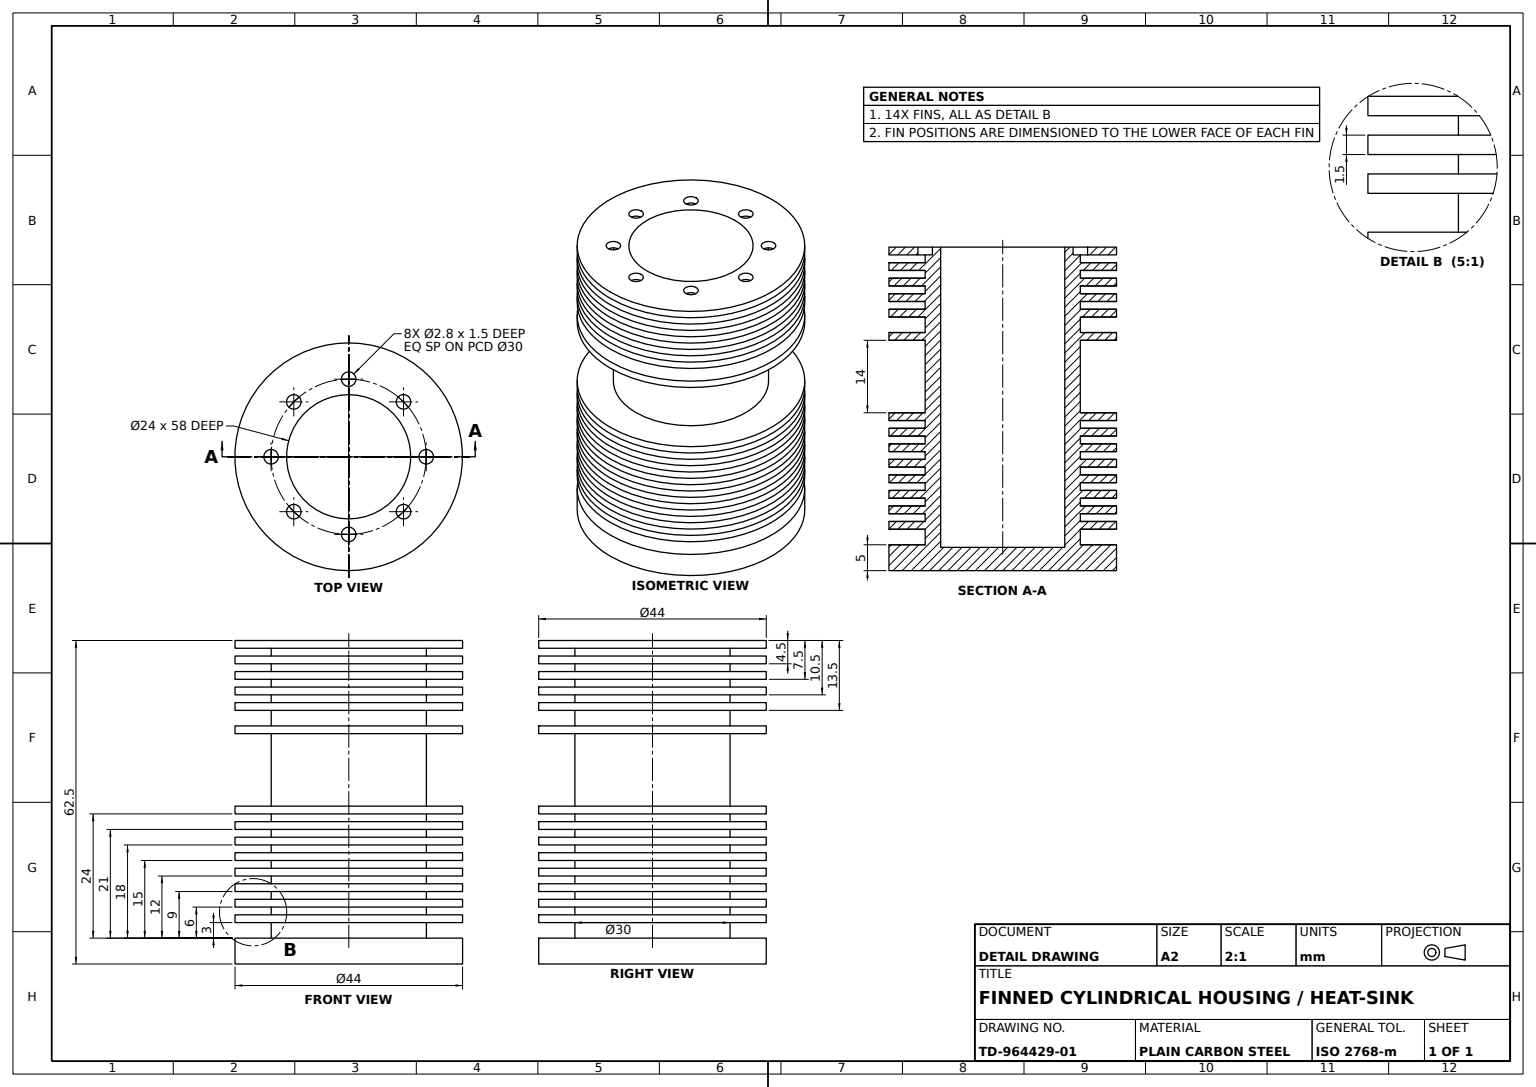
from build123d import *

# Parameters (mm, degrees)
BASE_DISC_SKETCH_R     = 22
BASE_DISC_DEPTH        = 5
LOWER_FIN_1_SKETCH_R   = 22
LOWER_FIN_1_DEPTH      = 1.5
LOWER_FIN_2_SKETCH_R   = 22
LOWER_FIN_2_DEPTH      = 1.5
LOWER_FIN_3_SKETCH_R   = 22
LOWER_FIN_3_DEPTH      = 1.5
LOWER_FIN_4_SKETCH_R   = 22
LOWER_FIN_4_DEPTH      = 1.5
LOWER_FIN_5_SKETCH_R   = 22
LOWER_FIN_5_DEPTH      = 1.5
LOWER_FIN_6_SKETCH_R   = 22
LOWER_FIN_6_DEPTH      = 1.5
LOWER_FIN_7_SKETCH_R   = 22
LOWER_FIN_7_DEPTH      = 1.5
LOWER_FIN_8_SKETCH_R   = 22
LOWER_FIN_8_DEPTH      = 1.5
UPPER_FIN_1_SKETCH_R   = 22
UPPER_FIN_1_DEPTH      = 1.5
UPPER_FIN_2_SKETCH_R   = 22
UPPER_FIN_2_DEPTH      = 1.5
UPPER_FIN_3_SKETCH_R   = 22
UPPER_FIN_3_DEPTH      = 1.5
UPPER_FIN_4_SKETCH_R   = 22
UPPER_FIN_4_DEPTH      = 1.5
UPPER_FIN_5_SKETCH_R   = 22
UPPER_FIN_5_DEPTH      = 1.5
UPPER_FIN_6_SKETCH_R   = 22
UPPER_FIN_6_DEPTH      = 1.5
CORE_BOSS_SKETCH_R     = 12
CORE_BOSS_58MM_DEPTH   = 58
HUB_BOSS_SKETCH_R      = 15
HUB_BOSS_58MM_DEPTH    = 58
CENTRAL_BORE_SKETCH_R  = 12
CENTRAL_BORE_DEPTH     = 58
BOLT_HOLES_8X_SKETCH_R = 1.4
BOLT_HOLES_8X_DEPTH    = 1.5


with BuildPart() as part:
    # Base Disc Sketch → Base Disc (new body)
    with BuildSketch(Plane(origin=(0, 0, 0), x_dir=(1, 0, 0), z_dir=(0, 1, 0))):
        with Locations(Location((0, 0, 0), (0, 0, 270))):
            Circle(BASE_DISC_SKETCH_R)
    extrude(amount=BASE_DISC_DEPTH)



with BuildPart() as body_2:
    # Lower Fin 1 Sketch → Lower Fin 1 (new body)
    with BuildSketch(Plane(origin=(0, 8, 0), x_dir=(1, 0, 0), z_dir=(0, 1, 0))):
        with Locations(Location((0, 0, 0), (0, 0, 270))):
            Circle(LOWER_FIN_1_SKETCH_R)
    extrude(amount=LOWER_FIN_1_DEPTH)


with BuildPart() as body_3:
    # Lower Fin 2 Sketch → Lower Fin 2 (new body)
    with BuildSketch(Plane(origin=(0, 11, 0), x_dir=(1, 0, 0), z_dir=(0, 1, 0))):
        with Locations(Location((0, 0, 0), (0, 0, 270))):
            Circle(LOWER_FIN_2_SKETCH_R)
    extrude(amount=LOWER_FIN_2_DEPTH)


with BuildPart() as body_4:
    # Lower Fin 3 Sketch → Lower Fin 3 (new body)
    with BuildSketch(Plane(origin=(0, 14, 0), x_dir=(1, 0, 0), z_dir=(0, 1, 0))):
        with Locations(Location((0, 0, 0), (0, 0, 270))):
            Circle(LOWER_FIN_3_SKETCH_R)
    extrude(amount=LOWER_FIN_3_DEPTH)


with BuildPart() as body_5:
    # Lower Fin 4 Sketch → Lower Fin 4 (new body)
    with BuildSketch(Plane(origin=(0, 17, 0), x_dir=(1, 0, 0), z_dir=(0, 1, 0))):
        with Locations(Location((0, 0, 0), (0, 0, 270))):
            Circle(LOWER_FIN_4_SKETCH_R)
    extrude(amount=LOWER_FIN_4_DEPTH)


with BuildPart() as body_6:
    # Lower Fin 5 Sketch → Lower Fin 5 (new body)
    with BuildSketch(Plane(origin=(0, 20, 0), x_dir=(1, 0, 0), z_dir=(0, 1, 0))):
        with Locations(Location((0, 0, 0), (0, 0, 270))):
            Circle(LOWER_FIN_5_SKETCH_R)
    extrude(amount=LOWER_FIN_5_DEPTH)


with BuildPart() as body_7:
    # Lower Fin 6 Sketch → Lower Fin 6 (new body)
    with BuildSketch(Plane(origin=(0, 23, 0), x_dir=(1, 0, 0), z_dir=(0, 1, 0))):
        with Locations(Location((0, 0, 0), (0, 0, 270))):
            Circle(LOWER_FIN_6_SKETCH_R)
    extrude(amount=LOWER_FIN_6_DEPTH)


with BuildPart() as body_8:
    # Lower Fin 7 Sketch → Lower Fin 7 (new body)
    with BuildSketch(Plane(origin=(0, 26, 0), x_dir=(1, 0, 0), z_dir=(0, 1, 0))):
        with Locations(Location((0, 0, 0), (0, 0, 270))):
            Circle(LOWER_FIN_7_SKETCH_R)
    extrude(amount=LOWER_FIN_7_DEPTH)


with BuildPart() as body_9:
    # Lower Fin 8 Sketch → Lower Fin 8 (new body)
    with BuildSketch(Plane(origin=(0, 29, 0), x_dir=(1, 0, 0), z_dir=(0, 1, 0))):
        with Locations(Location((0, 0, 0), (0, 0, 270))):
            Circle(LOWER_FIN_8_SKETCH_R)
    extrude(amount=LOWER_FIN_8_DEPTH)


with BuildPart() as body_10:
    # Upper Fin 1 Sketch → Upper Fin 1 (new body)
    with BuildSketch(Plane(origin=(0, 44.5, 0), x_dir=(1, 0, 0), z_dir=(0, 1, 0))):
        with Locations(Location((0, 0, 0), (0, 0, 270))):
            Circle(UPPER_FIN_1_SKETCH_R)
    extrude(amount=UPPER_FIN_1_DEPTH)


with BuildPart() as body_11:
    # Upper Fin 2 Sketch → Upper Fin 2 (new body)
    with BuildSketch(Plane(origin=(0, 49, 0), x_dir=(1, 0, 0), z_dir=(0, 1, 0))):
        with Locations(Location((0, 0, 0), (0, 0, 270))):
            Circle(UPPER_FIN_2_SKETCH_R)
    extrude(amount=UPPER_FIN_2_DEPTH)


with BuildPart() as body_12:
    # Upper Fin 3 Sketch → Upper Fin 3 (new body)
    with BuildSketch(Plane(origin=(0, 52, 0), x_dir=(1, 0, 0), z_dir=(0, 1, 0))):
        with Locations(Location((0, 0, 0), (0, 0, 270))):
            Circle(UPPER_FIN_3_SKETCH_R)
    extrude(amount=UPPER_FIN_3_DEPTH)


with BuildPart() as body_13:
    # Upper Fin 4 Sketch → Upper Fin 4 (new body)
    with BuildSketch(Plane(origin=(0, 55, 0), x_dir=(1, 0, 0), z_dir=(0, 1, 0))):
        with Locations(Location((0, 0, 0), (0, 0, 270))):
            Circle(UPPER_FIN_4_SKETCH_R)
    extrude(amount=UPPER_FIN_4_DEPTH)


with BuildPart() as body_14:
    # Upper Fin 5 Sketch → Upper Fin 5 (new body)
    with BuildSketch(Plane(origin=(0, 58, 0), x_dir=(1, 0, 0), z_dir=(0, 1, 0))):
        with Locations(Location((0, 0, 0), (0, 0, 270))):
            Circle(UPPER_FIN_5_SKETCH_R)
    extrude(amount=UPPER_FIN_5_DEPTH)


with BuildPart() as body_15:
    # Upper Fin 6 Sketch → Upper Fin 6 (new body)
    with BuildSketch(Plane(origin=(0, 61, 0), x_dir=(1, 0, 0), z_dir=(0, 1, 0))):
        with Locations(Location((0, 0, 0), (0, 0, 270))):
            Circle(UPPER_FIN_6_SKETCH_R)
    extrude(amount=UPPER_FIN_6_DEPTH)


with BuildPart() as part_1:
    add(part.part)

    add(body_2.part)  # Core Boss 58mm merges body 2

    add(body_3.part)  # Core Boss 58mm merges body 3

    add(body_4.part)  # Core Boss 58mm merges body 4

    add(body_5.part)  # Core Boss 58mm merges body 5

    add(body_6.part)  # Core Boss 58mm merges body 6

    add(body_7.part)  # Core Boss 58mm merges body 7

    add(body_8.part)  # Core Boss 58mm merges body 8

    add(body_9.part)  # Core Boss 58mm merges body 9

    add(body_10.part)  # Core Boss 58mm merges body 10

    add(body_11.part)  # Core Boss 58mm merges body 11

    add(body_12.part)  # Core Boss 58mm merges body 12

    add(body_13.part)  # Core Boss 58mm merges body 13

    add(body_14.part)  # Core Boss 58mm merges body 14

    add(body_15.part)  # Core Boss 58mm merges body 15
    # Core Boss Sketch → Core Boss 58mm (add)
    with BuildSketch(Plane(origin=(0, 62.5, 0), x_dir=(1, 0, 0), z_dir=(0, 1, 0))):
        with Locations(Location((0, 0, 0), (0, 0, 270))):
            Circle(CORE_BOSS_SKETCH_R)
    extrude(amount=-CORE_BOSS_58MM_DEPTH)

    # Hub Boss Sketch → Hub Boss 58mm (add)
    with BuildSketch(Plane(origin=(0, 62.5, 0), x_dir=(1, 0, 0), z_dir=(0, 1, 0))):
        with Locations(Location((0, 0, 0), (0, 0, 270))):
            Circle(HUB_BOSS_SKETCH_R)
    extrude(amount=-HUB_BOSS_58MM_DEPTH)

    # Central Bore Sketch → Central Bore (cut)
    with BuildSketch(Plane(origin=(0, 62.5, 0), x_dir=(1, 0, 0), z_dir=(0, 1, 0))):
        with Locations(Location((0, 0, 0), (0, 0, 270))):
            Circle(CENTRAL_BORE_SKETCH_R)
    extrude(amount=-CENTRAL_BORE_DEPTH, mode=Mode.SUBTRACT)

    # Bolt Holes 8x Sketch → Bolt Holes 8x (cut)
    with BuildSketch(Plane(origin=(0, 62.5, 0), x_dir=(1, 0, 0), z_dir=(0, 1, 0))):
        with Locations(Location((0, 15, 0), (0, 0, 270))):
            Circle(BOLT_HOLES_8X_SKETCH_R)
        with Locations(Location((10.606601718, 10.606601718, 0), (0, 0, 270))):
            Circle(BOLT_HOLES_8X_SKETCH_R)
        with Locations(Location((15, 0, 0), (0, 0, 270))):
            Circle(BOLT_HOLES_8X_SKETCH_R)
        with Locations(Location((10.606601718, -10.606601718, 0), (0, 0, 270))):
            Circle(BOLT_HOLES_8X_SKETCH_R)
        with Locations(Location((0, -15, 0), (0, 0, 270))):
            Circle(BOLT_HOLES_8X_SKETCH_R)
        with Locations(Location((-10.606601718, -10.606601718, 0), (0, 0, 270))):
            Circle(BOLT_HOLES_8X_SKETCH_R)
        with Locations(Location((-15, 0, 0), (0, 0, 270))):
            Circle(BOLT_HOLES_8X_SKETCH_R)
        with Locations(Location((-10.606601718, 10.606601718, 0), (0, 0, 270))):
            Circle(BOLT_HOLES_8X_SKETCH_R)
    extrude(amount=-BOLT_HOLES_8X_DEPTH, mode=Mode.SUBTRACT)


solid = part_1.part
